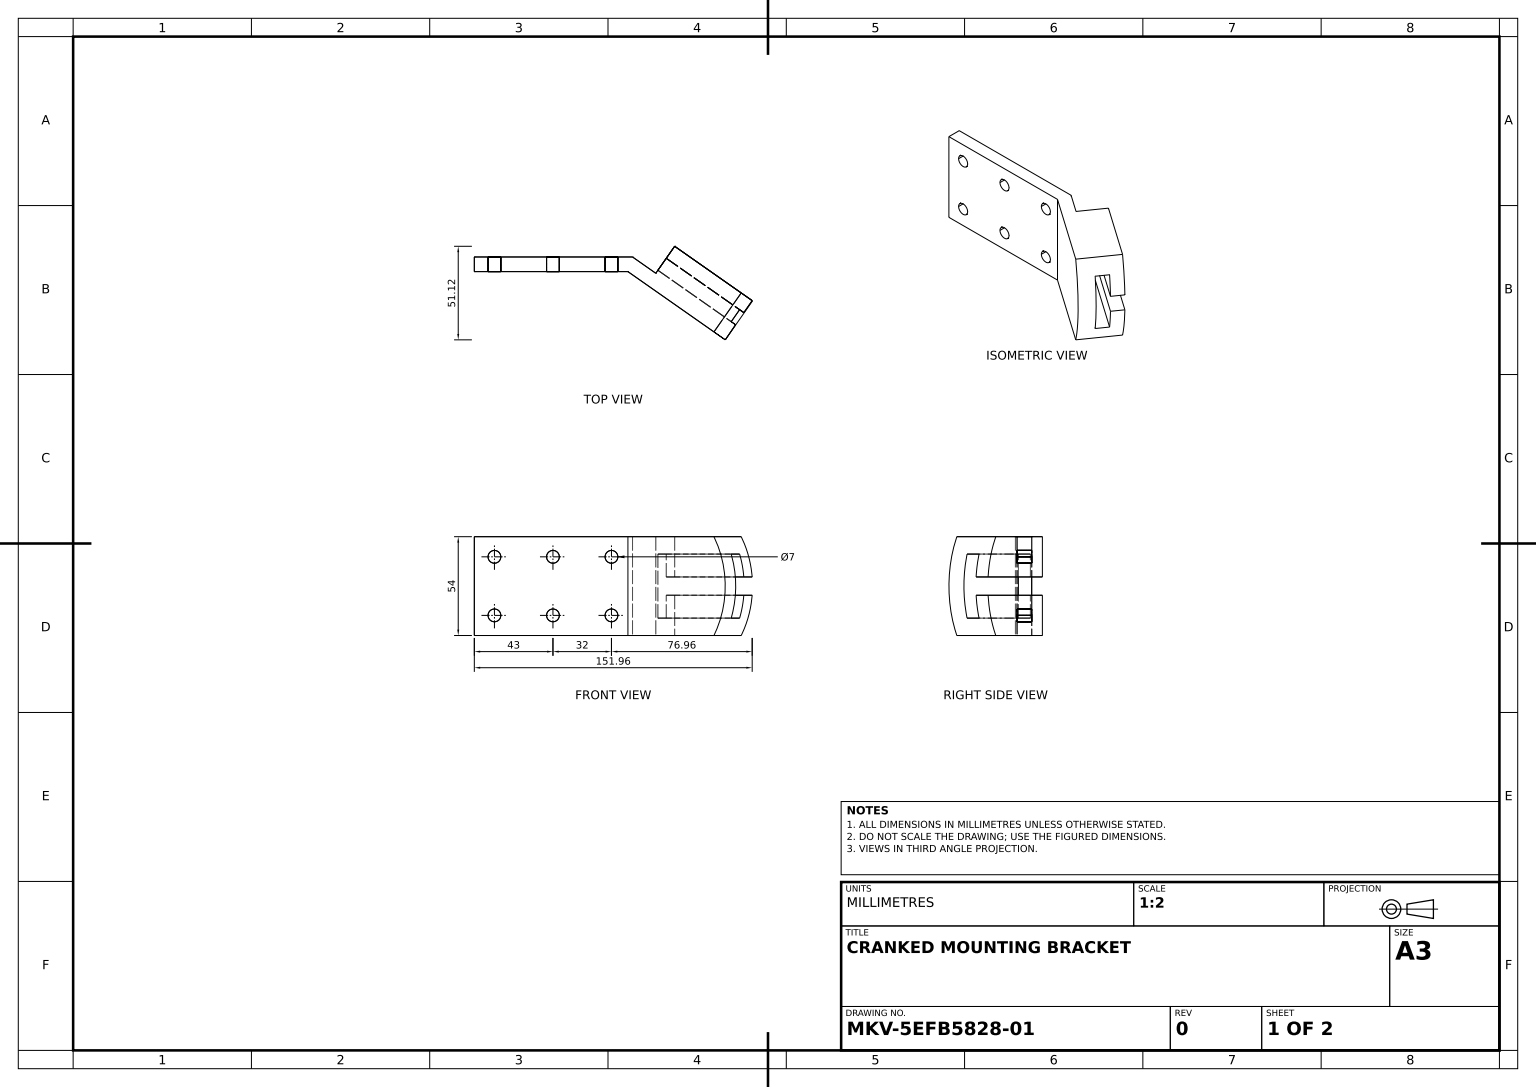
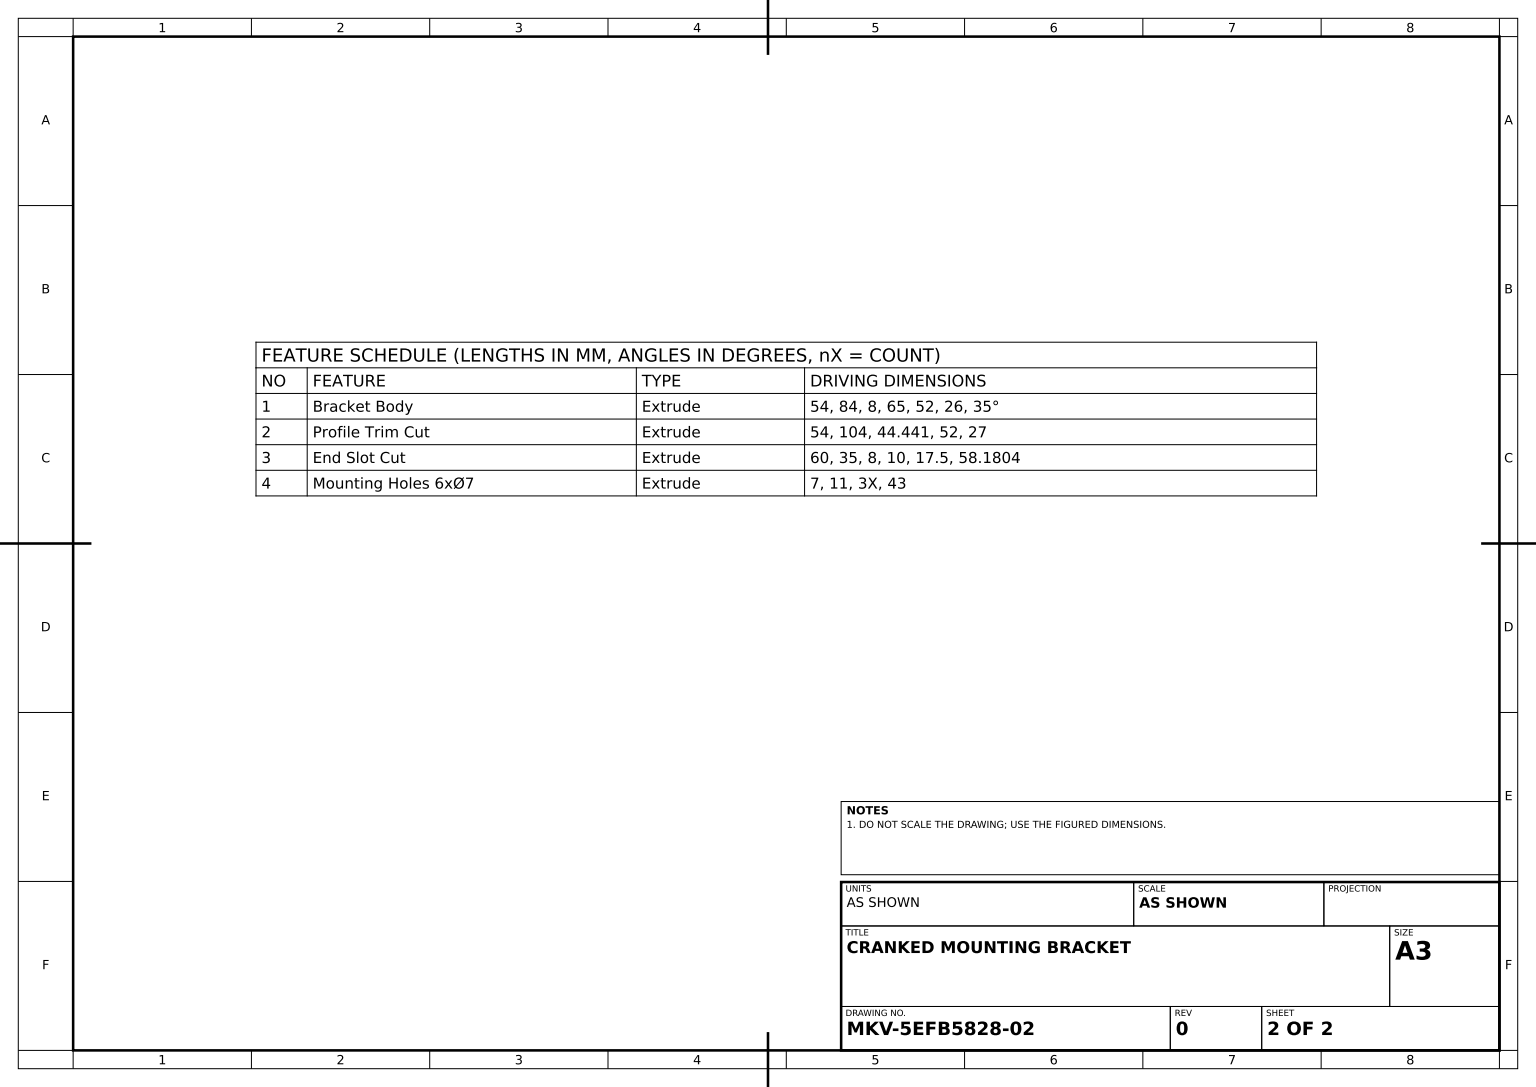
from build123d import *

# Parameters (mm, degrees)
BRACKET_BODY_DEPTH        = 27
PROFILE_TRIM_CUT_DEPTH    = 54
END_SLOT_CUT_DEPTH        = 60
MOUNTING_HOLES_SKETCH_R   = 3.5
MOUNTING_HOLES_6X_7_DEPTH = 8


with BuildPart() as part:
    # Bracket Profile Sketch → Bracket Body (new, symmetric)
    with BuildSketch(Plane(origin=(0, 0, 0), x_dir=(1, 0, 0), z_dir=(0, 1, 0))):
        Polygon((0, 0), (0, 8), (86.522390311, 8), (99.237588067, -0.903277318), (109.561963921, 13.841459479), (152.157870224, -15.984515211), (137.244882879, -37.282468363), (84, 0), align=None)
    extrude(amount=BRACKET_BODY_DEPTH, both=True)

    # Profile Trim Sketch → Profile Trim Cut (cut)
    with BuildSketch(Plane(origin=(42.548141325, 0, -60.765043225), x_dir=(-0.819152044288991, 0, -0.5735764363510474), z_dir=(0.5735764363510474, 0, -0.819152044288991))):
        with BuildLine():
            ThreePointArc((-133.80877172, 1.36e-07), (-131.883368797, 14.019084406), (-126.249743807, 27))
            Line((-126.249743807, 27), (-133.80877172, 27))
            Line((-133.80877172, 27), (-133.80877172, 1.36e-07))
        make_face()
        with BuildLine():
            ThreePointArc((-126.249743807, -27), (-131.883368834, -14.019084275), (-133.80877172, 1.36e-07))
            Line((-133.80877172, 1.36e-07), (-133.80877172, -27))
            Line((-133.80877172, -27), (-126.249743807, -27))
        make_face()
    extrude(amount=-PROFILE_TRIM_CUT_DEPTH, mode=Mode.SUBTRACT)

    # End Slot Sketch → End Slot Cut (cut)
    with BuildSketch(Plane(origin=(116.162945253, 0, 81.338169927), x_dir=(-0.5735764363510482, 0, 0.8191520442889904), z_dir=(-0.8191520442889904, 0, -0.5735764363510482))):
        Polygon((-74.180420653, 5), (-66.180420653, 5), (-66.180420653, 17.5), (-58.180420653, 17.5), (-58.180420653, -17.5), (-66.180420653, -17.5), (-66.180420653, -5), (-74.180420653, -5), align=None)
    extrude(amount=END_SLOT_CUT_DEPTH, mode=Mode.SUBTRACT)

    # Mounting Holes Sketch → Mounting Holes 6xØ7 (cut)
    with BuildSketch(Plane(origin=(0, 0, -8), x_dir=(-1, 0, 0), z_dir=(0, 0, -1))):
        with Locations((-11, 16)):
            Circle(MOUNTING_HOLES_SKETCH_R)
        with Locations((-11, -16)):
            Circle(MOUNTING_HOLES_SKETCH_R)
        with Locations((-43, 16)):
            Circle(MOUNTING_HOLES_SKETCH_R)
        with Locations((-43, -16)):
            Circle(MOUNTING_HOLES_SKETCH_R)
        with Locations((-75, 16)):
            Circle(MOUNTING_HOLES_SKETCH_R)
        with Locations((-75, -16)):
            Circle(MOUNTING_HOLES_SKETCH_R)
    extrude(amount=-MOUNTING_HOLES_6X_7_DEPTH, mode=Mode.SUBTRACT)


solid = part.part
